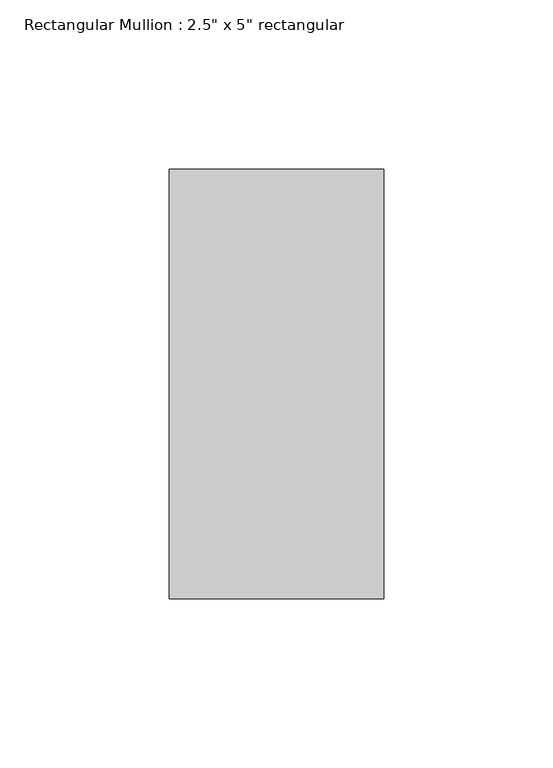
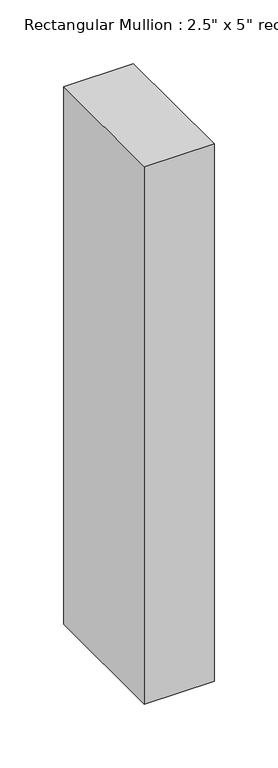
"""IFC4 building model written with IfcOpenShell, lengths in millimetres: member geometry."""

from ifc_helpers import new_model, si_unit, frame, origin, place, context, project, spatial, polyline, outline, extrude, source, transform, mapped, element, save


def member_b3098cb3(model_context):
    return source(origin(), model_context, "Body", "SweptSolid", [
        extrude(outline(polyline([(31.75, 63.5), (31.75, -63.5), (-31.75, -63.5), (-31.75, 63.5), (31.75, 63.5)])), frame((0.0, 0.0, -516.4666667), z_axis=(0.0, 0.0, 1.0), x_axis=(1.0, 0.0, 0.0)), (0.0, 0.0, 1.0), 516.4666667),
    ])


if __name__ == "__main__":
    model = new_model("IFC4")
    model_context = context("Model", 3, world=origin())
    ifc_project = project(units=[si_unit("LENGTHUNIT", "METRE", prefix="MILLI")], contexts=[model_context])
    site = spatial("IfcSite", under=ifc_project)
    building = spatial("IfcBuilding", under=site)
    placement = place(None, origin())
    member_shape = member_b3098cb3(model_context)
    element("IfcMember", 1, ObjectType="Rectangular Mullion : 2.5\" x 5\" rectangular", at=placement, inside=building, context=model_context, shape_type="MappedRepresentation", body=[
        mapped(member_shape, transform((0.0, 0.0, 0.0), x_axis=(1.0, 0.0, 0.0), y_axis=(0.0, 1.0, 0.0), z_axis=(0.0, 0.0, 1.0))),
    ])
    save(model, "model.ifc")

# Revit data of these elements
# Type "Rectangular Mullion : 2.5\" x 5\" rectangular"
#   built-in parameter 1007304 = 0.416667 (stored number, unit not read)
#   built-in parameter 1007301 = 0.104167 (stored number, unit not read)
#   built-in parameter 1007300 = 0.104167 (stored number, unit not read)
# Element 1 (IfcMember, "Rectangular Mullion : 2.5\" x 5\" rectangular")
#   Materials on its faces: "Aluminum"
# Materials
#   "Aluminum": class "Metal", colour RGB 247 247 247, transparency 0, Description = "Aluminum 6061", Cost = 0
